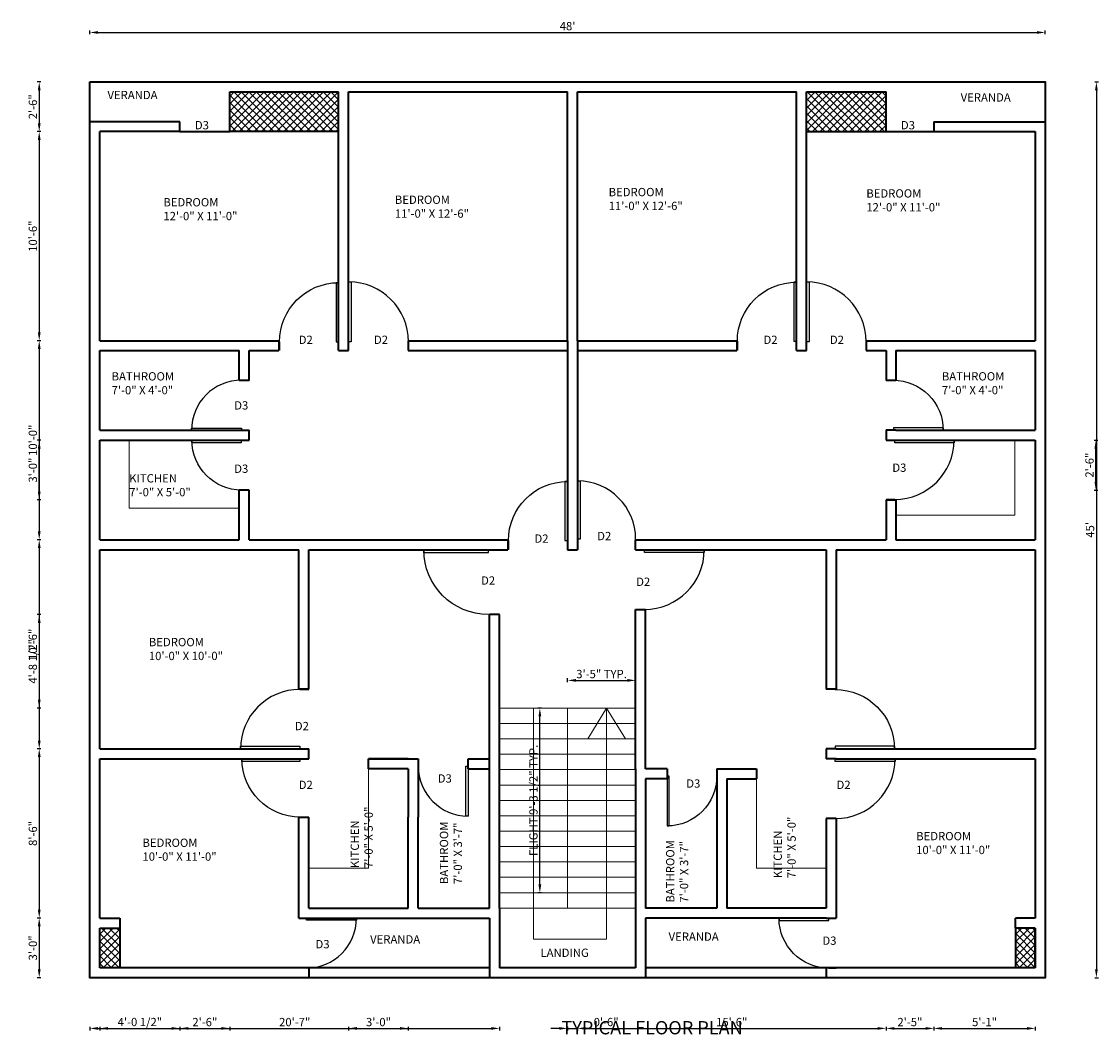
# Model space of a CAD drawing. Units: inches. Extents: x -42 to 607, y -560 to 51.
import ezdxf

# ---------------------------------------------------------------- set-up
doc = ezdxf.new("R2010")
doc.units = ezdxf.units.IN
for name, color, linetype, lineweight in [('A-ANNO-DIMS', 2, 'Continuous', 18), ('A-ANNO-SYMB', 7, 'Continuous', 18), ('A-ANNO-TEXT', 7, 'Continuous', 35), ('A-AREA-IDEN', 7, 'Continuous', 18), ('A-DOOR', 3, 'Continuous', 25), ('A-DOOR-IDEN', 3, 'Continuous', 18), ('A-FLOR-FIXT', 9, 'Continuous', 18), ('A-FLOR-STRS', 4, 'Continuous', 18), ('A-WALL', 7, 'Continuous', 35), ('A-WALL-PATT', 28, 'Continuous', 13)]:
    doc.layers.add(name, color=color, linetype=linetype, lineweight=lineweight)
doc.styles.get("Standard").update_dxf_attribs({"font": 'arial.ttf'})
doc.dimstyles.new('ISO-25', dxfattribs={"dimtxt": 5, "dimasz": 5, "dimexe": 1.25, "dimexo": 0.625, "dimtad": 1, "dimlunit": 3, "dimtxsty": 'Standard', "dimcen": 2.5, "dimadec": 0, "dimazin": 0, "dimtfac": 1, "dimtmove": 0, "dimatfit": 3, "dimfxl": 1, "dimfxlon": 1, "dimarcsym": 0})

# ---------------------------------------------------------------- blocks, each defined once
blk = doc.blocks.new('*U2')
for p, q in [((0, 0), (0, -6)), ((40, 0), (40, -6))]:
    blk.add_line(p, q)
blk.add_lwpolyline([(0, 0), (0, 40), (1.75, 40), (1.75, 0)], close=True)
blk.add_arc((0, 0), 40, 0, 90)
blk = doc.blocks.new('*D3')
at = {"layer": 'A-ANNO-DIMS', "color": 0, "lineweight": -2, "transparency": 16777216}
for p, q in [((-1, 43.9), (-1, 46.15)), ((575, 43.9), (575, 46.15)), ((4, 44.9), (570, 44.9))]:
    blk.add_line(p, q, dxfattribs=at)
at = {"layer": 'A-ANNO-DIMS', "color": 0, "transparency": 16777216}
for points in [[(4, 45.73), (4, 44.07), (-1, 44.9)], [(570, 45.73), (570, 44.07), (575, 44.9)]]:
    blk.add_solid(points, dxfattribs=at)
at = {"layer": 'Defpoints', "color": 0, "transparency": 16777216}
for p in [(575, 44.9), (-1, 15.11), (575, 15.11)]:
    blk.add_point(p, dxfattribs=at)
at = {"layer": 'A-ANNO-DIMS', "color": 0, "transparency": 16777216, "insert": (287, 48.08), "char_height": 5, "attachment_point": 5}
blk.add_mtext("48'", dxfattribs=at)
blk = doc.blocks.new('*D4')
at = {"layer": 'A-ANNO-DIMS', "color": 0, "lineweight": -2, "transparency": 16777216}
for p, q in [((604.84, 15.11), (607.09, 15.11)), ((605.84, 10.11), (605.84, -519.89)), ((604.84, -524.89), (607.09, -524.89))]:
    blk.add_line(p, q, dxfattribs=at)
at = {"layer": 'A-ANNO-DIMS', "color": 0, "transparency": 16777216}
for points in [[(605.01, 10.11), (606.67, 10.11), (605.84, 15.11)], [(605.01, -519.89), (606.67, -519.89), (605.84, -524.89)]]:
    blk.add_solid(points, dxfattribs=at)
at = {"layer": 'Defpoints', "color": 0, "transparency": 16777216}
for p in [(575, 15.11), (575, -524.89), (605.84, -524.89)]:
    blk.add_point(p, dxfattribs=at)
at = {"layer": 'A-ANNO-DIMS', "color": 0, "transparency": 16777216, "insert": (602.67, -254.89), "char_height": 5, "attachment_point": 5, "rotation": 90}
blk.add_mtext("45'", dxfattribs=at)
blk = doc.blocks.new('STAIR-FLIGHT-41IN')
for p, q in [((41, 111.29), (0, 111.29)), ((41, 102.01), (0, 102.01)), ((41, 92.74), (0, 92.74)), ((41, 83.46), (0, 83.46)), ((41, 74.19), (0, 74.19)), ((41, 64.92), (0, 64.92)), ((41, 55.64), (0, 55.64)), ((41, 46.37), (0, 46.37)), ((41, 37.1), (0, 37.1)), ((41, 27.82), (0, 27.82)), ((41, 18.55), (0, 18.55)), ((41, 9.27), (0, 9.27)), ((41, 0), (0, 0))]:
    blk.add_line(p, q)
blk = doc.blocks.new('*D6')
at = {"layer": 'A-ANNO-DIMS', "color": 0, "lineweight": -2, "transparency": 16777216}
for p, q in [((271.31, -362.33), (269.06, -362.33)), ((270.31, -468.61), (270.31, -367.33)), ((271.31, -473.61), (269.06, -473.61))]:
    blk.add_line(p, q, dxfattribs=at)
at = {"layer": 'A-ANNO-DIMS', "color": 0, "transparency": 16777216}
for points in [[(269.47, -367.33), (271.14, -367.33), (270.31, -362.33)], [(269.47, -468.61), (271.14, -468.61), (270.31, -473.61)]]:
    blk.add_solid(points, dxfattribs=at)
at = {"layer": 'Defpoints', "color": 0, "transparency": 16777216}
for p in [(270.31, -362.33), (287, -362.33), (287, -473.61)]:
    blk.add_point(p, dxfattribs=at)
at = {"layer": 'A-ANNO-DIMS', "color": 0, "transparency": 16777216, "insert": (267.1, -417.97), "char_height": 5, "attachment_point": 5, "rotation": 90}
blk.add_mtext('FLIGHT 9\'-3 1/2" TYP.', dxfattribs=at)
blk = doc.blocks.new('*D7')
at = {"layer": 'A-ANNO-DIMS', "color": 0, "lineweight": -2, "transparency": 16777216}
for p, q in [((287, -346.64), (287, -344.39)), ((292, -345.64), (323, -345.64)), ((328, -346.64), (328, -344.39))]:
    blk.add_line(p, q, dxfattribs=at)
at = {"layer": 'A-ANNO-DIMS', "color": 0, "transparency": 16777216}
for points in [[(292, -344.8), (292, -346.47), (287, -345.64)], [(323, -344.8), (323, -346.47), (328, -345.64)]]:
    blk.add_solid(points, dxfattribs=at)
at = {"layer": 'Defpoints', "color": 0, "transparency": 16777216}
for p in [(328, -345.64), (287, -362.33), (328, -362.33)]:
    blk.add_point(p, dxfattribs=at)
at = {"layer": 'A-ANNO-DIMS', "color": 0, "transparency": 16777216, "insert": (307.5, -342.46), "char_height": 5, "attachment_point": 5}
blk.add_mtext('3\'-5" TYP.', dxfattribs=at)
blk = doc.blocks.new('*D8')
at = {"layer": 'A-ANNO-DIMS', "color": 0, "lineweight": -2, "transparency": 16777216}
for p, q in [((-30.52, 15.11), (-32.77, 15.11)), ((-31.52, 10.11), (-31.52, -9.89)), ((-30.52, -14.89), (-32.77, -14.89))]:
    blk.add_line(p, q, dxfattribs=at)
at = {"layer": 'A-ANNO-DIMS', "color": 0, "transparency": 16777216}
for points in [[(-32.35, 10.11), (-30.69, 10.11), (-31.52, 15.11)], [(-32.35, -9.89), (-30.69, -9.89), (-31.52, -14.89)]]:
    blk.add_solid(points, dxfattribs=at)
at = {"layer": 'Defpoints', "color": 0, "transparency": 16777216}
for p in [(-1, 15.11), (-31.52, -14.89), (5, -14.89)]:
    blk.add_point(p, dxfattribs=at)
at = {"layer": 'A-ANNO-DIMS', "color": 0, "transparency": 16777216, "insert": (-34.7, 0.11), "char_height": 5, "attachment_point": 5, "rotation": 90}
blk.add_mtext('2\'-6"', dxfattribs=at)
blk = doc.blocks.new('*D9')
at = {"layer": 'A-ANNO-DIMS', "color": 0, "lineweight": -2, "transparency": 16777216}
for p, q in [((-30.52, -14.89), (-32.77, -14.89)), ((-31.52, -19.89), (-31.52, -135.89)), ((-30.52, -140.89), (-32.77, -140.89))]:
    blk.add_line(p, q, dxfattribs=at)
at = {"layer": 'A-ANNO-DIMS', "color": 0, "transparency": 16777216}
for points in [[(-32.35, -19.89), (-30.69, -19.89), (-31.52, -14.89)], [(-32.35, -135.89), (-30.69, -135.89), (-31.52, -140.89)]]:
    blk.add_solid(points, dxfattribs=at)
at = {"layer": 'Defpoints', "color": 0, "transparency": 16777216}
for p in [(5, -14.89), (-31.52, -140.89), (5, -140.89)]:
    blk.add_point(p, dxfattribs=at)
at = {"layer": 'A-ANNO-DIMS', "color": 0, "transparency": 16777216, "insert": (-34.7, -77.89), "char_height": 5, "attachment_point": 5, "rotation": 90}
blk.add_mtext('10\'-6"', dxfattribs=at)
blk = doc.blocks.new('*D10')
at = {"layer": 'A-ANNO-DIMS', "color": 0, "lineweight": -2, "transparency": 16777216}
for p, q in [((-30.52, -140.89), (-32.77, -140.89)), ((-31.52, -145.89), (-31.52, -255.89)), ((-30.52, -260.89), (-32.77, -260.89))]:
    blk.add_line(p, q, dxfattribs=at)
at = {"layer": 'A-ANNO-DIMS', "color": 0, "transparency": 16777216}
for points in [[(-32.35, -145.89), (-30.69, -145.89), (-31.52, -140.89)], [(-32.35, -255.89), (-30.69, -255.89), (-31.52, -260.89)]]:
    blk.add_solid(points, dxfattribs=at)
at = {"layer": 'Defpoints', "color": 0, "transparency": 16777216}
for p in [(5, -140.89), (-31.52, -260.89), (5, -260.89)]:
    blk.add_point(p, dxfattribs=at)
at = {"layer": 'A-ANNO-DIMS', "color": 0, "transparency": 16777216, "insert": (-34.7, -200.89), "char_height": 5, "attachment_point": 5, "rotation": 90}
blk.add_mtext('10\'-0"', dxfattribs=at)
blk = doc.blocks.new('*D11')
at = {"layer": 'A-ANNO-DIMS', "color": 0, "lineweight": -2, "transparency": 16777216}
for p, q in [((-30.52, -260.89), (-32.77, -260.89)), ((-31.52, -265.89), (-31.52, -381.89)), ((-30.52, -386.89), (-32.77, -386.89))]:
    blk.add_line(p, q, dxfattribs=at)
at = {"layer": 'A-ANNO-DIMS', "color": 0, "transparency": 16777216}
for points in [[(-32.35, -265.89), (-30.69, -265.89), (-31.52, -260.89)], [(-32.35, -381.89), (-30.69, -381.89), (-31.52, -386.89)]]:
    blk.add_solid(points, dxfattribs=at)
at = {"layer": 'Defpoints', "color": 0, "transparency": 16777216}
for p in [(5, -260.89), (-31.52, -386.89), (5, -386.89)]:
    blk.add_point(p, dxfattribs=at)
at = {"layer": 'A-ANNO-DIMS', "color": 0, "transparency": 16777216, "insert": (-34.7, -323.89), "char_height": 5, "attachment_point": 5, "rotation": 90}
blk.add_mtext('10\'-6"', dxfattribs=at)
blk = doc.blocks.new('*D12')
at = {"layer": 'A-ANNO-DIMS', "color": 0, "lineweight": -2, "transparency": 16777216}
for p, q in [((-30.52, -386.89), (-32.77, -386.89)), ((-31.52, -391.89), (-31.52, -483.89)), ((-30.52, -488.89), (-32.77, -488.89))]:
    blk.add_line(p, q, dxfattribs=at)
at = {"layer": 'A-ANNO-DIMS', "color": 0, "transparency": 16777216}
for points in [[(-32.35, -391.89), (-30.69, -391.89), (-31.52, -386.89)], [(-32.35, -483.89), (-30.69, -483.89), (-31.52, -488.89)]]:
    blk.add_solid(points, dxfattribs=at)
at = {"layer": 'Defpoints', "color": 0, "transparency": 16777216}
for p in [(5, -386.89), (-31.52, -488.89), (5, -488.89)]:
    blk.add_point(p, dxfattribs=at)
at = {"layer": 'A-ANNO-DIMS', "color": 0, "transparency": 16777216, "insert": (-34.7, -437.89), "char_height": 5, "attachment_point": 5, "rotation": 90}
blk.add_mtext('8\'-6"', dxfattribs=at)
blk = doc.blocks.new('*D13')
at = {"layer": 'A-ANNO-DIMS', "color": 0, "lineweight": -2, "transparency": 16777216}
for p, q in [((-30.52, -488.89), (-32.77, -488.89)), ((-31.52, -493.89), (-31.52, -519.89)), ((-30.52, -524.89), (-32.77, -524.89))]:
    blk.add_line(p, q, dxfattribs=at)
at = {"layer": 'A-ANNO-DIMS', "color": 0, "transparency": 16777216}
for points in [[(-32.35, -493.89), (-30.69, -493.89), (-31.52, -488.89)], [(-32.35, -519.89), (-30.69, -519.89), (-31.52, -524.89)]]:
    blk.add_solid(points, dxfattribs=at)
at = {"layer": 'Defpoints', "color": 0, "transparency": 16777216}
for p in [(5, -488.89), (-31.52, -524.89), (-1, -524.89)]:
    blk.add_point(p, dxfattribs=at)
at = {"layer": 'A-ANNO-DIMS', "color": 0, "transparency": 16777216, "insert": (-34.7, -506.89), "char_height": 5, "attachment_point": 5, "rotation": 90}
blk.add_mtext('3\'-0"', dxfattribs=at)
blk = doc.blocks.new('*D14')
at = {"layer": 'A-ANNO-DIMS', "color": 0, "lineweight": -2, "transparency": 16777216}
for p, q in [((-1, -554.41), (-1, -556.66)), ((4, -555.41), (241, -555.41)), ((246, -554.41), (246, -556.66))]:
    blk.add_line(p, q, dxfattribs=at)
at = {"layer": 'A-ANNO-DIMS', "color": 0, "transparency": 16777216}
for points in [[(4, -554.58), (4, -556.24), (-1, -555.41)], [(241, -554.58), (241, -556.24), (246, -555.41)]]:
    blk.add_solid(points, dxfattribs=at)
at = {"layer": 'Defpoints', "color": 0, "transparency": 16777216}
for p in [(246, -518.89), (-1, -524.89), (246, -555.41)]:
    blk.add_point(p, dxfattribs=at)
at = {"layer": 'A-ANNO-DIMS', "color": 0, "transparency": 16777216, "insert": (122.5, -552.23), "char_height": 5, "attachment_point": 5}
blk.add_mtext('20\'-7"', dxfattribs=at)
blk = doc.blocks.new('*D15')
at = {"layer": 'A-ANNO-DIMS', "color": 0, "lineweight": -2, "transparency": 16777216}
for p, q in [((-30.52, -306.02), (-32.77, -306.02)), ((-31.52, -311.02), (-31.52, -357.33)), ((-30.52, -362.33), (-32.77, -362.33))]:
    blk.add_line(p, q, dxfattribs=at)
at = {"layer": 'A-ANNO-DIMS', "color": 0, "transparency": 16777216}
for points in [[(-32.35, -311.02), (-30.69, -311.02), (-31.52, -306.02)], [(-32.35, -357.33), (-30.69, -357.33), (-31.52, -362.33)]]:
    blk.add_solid(points, dxfattribs=at)
at = {"layer": 'Defpoints', "color": 0, "transparency": 16777216}
for p in [(240, -306.02), (-31.52, -362.33), (246, -362.33)]:
    blk.add_point(p, dxfattribs=at)
at = {"layer": 'A-ANNO-DIMS', "color": 0, "transparency": 16777216, "insert": (-34.73, -334.17), "char_height": 5, "attachment_point": 5, "rotation": 90}
blk.add_mtext('4\'-8 1/2"', dxfattribs=at)
blk = doc.blocks.new('*D16')
at = {"layer": 'A-ANNO-DIMS', "color": 0, "lineweight": -2, "transparency": 16777216}
for p, q in [((5, -554.41), (5, -556.66)), ((10, -555.41), (48.34, -555.41)), ((53.34, -554.41), (53.34, -556.66))]:
    blk.add_line(p, q, dxfattribs=at)
at = {"layer": 'A-ANNO-DIMS', "color": 0, "transparency": 16777216}
for points in [[(10, -554.58), (10, -556.24), (5, -555.41)], [(48.34, -554.58), (48.34, -556.24), (53.34, -555.41)]]:
    blk.add_solid(points, dxfattribs=at)
at = {"layer": 'Defpoints', "color": 0, "transparency": 16777216}
for p in [(5, -14.89), (53.34, -14.89), (53.34, -555.41)]:
    blk.add_point(p, dxfattribs=at)
at = {"layer": 'A-ANNO-DIMS', "color": 0, "transparency": 16777216, "insert": (29.17, -552.2), "char_height": 5, "attachment_point": 5}
blk.add_mtext('4\'-0 1/2"', dxfattribs=at)
blk = doc.blocks.new('*D17')
at = {"layer": 'A-ANNO-DIMS', "color": 0, "lineweight": -2, "transparency": 16777216}
for p, q in [((53.34, -554.41), (53.34, -556.66)), ((58.34, -555.41), (78.34, -555.41)), ((83.34, -554.41), (83.34, -556.66))]:
    blk.add_line(p, q, dxfattribs=at)
at = {"layer": 'A-ANNO-DIMS', "color": 0, "transparency": 16777216}
for points in [[(58.34, -554.58), (58.34, -556.24), (53.34, -555.41)], [(78.34, -554.58), (78.34, -556.24), (83.34, -555.41)]]:
    blk.add_solid(points, dxfattribs=at)
at = {"layer": 'Defpoints', "color": 0, "transparency": 16777216}
for p in [(53.34, -14.89), (83.34, -14.89), (83.34, -555.41)]:
    blk.add_point(p, dxfattribs=at)
at = {"layer": 'A-ANNO-DIMS', "color": 0, "transparency": 16777216, "insert": (68.34, -552.23), "char_height": 5, "attachment_point": 5}
blk.add_mtext('2\'-6"', dxfattribs=at)
blk = doc.blocks.new('*D18')
at = {"layer": 'A-ANNO-DIMS', "color": 0, "lineweight": -2, "transparency": 16777216}
for p, q in [((507.85, -554.41), (507.85, -556.66)), ((512.85, -555.41), (564, -555.41)), ((569, -554.41), (569, -556.66))]:
    blk.add_line(p, q, dxfattribs=at)
at = {"layer": 'A-ANNO-DIMS', "color": 0, "transparency": 16777216}
for points in [[(512.85, -554.58), (512.85, -556.24), (507.85, -555.41)], [(564, -554.58), (564, -556.24), (569, -555.41)]]:
    blk.add_solid(points, dxfattribs=at)
at = {"layer": 'Defpoints', "color": 0, "transparency": 16777216}
for p in [(507.85, -14.89), (569, -14.89), (569, -555.41)]:
    blk.add_point(p, dxfattribs=at)
at = {"layer": 'A-ANNO-DIMS', "color": 0, "transparency": 16777216, "insert": (538.42, -552.23), "char_height": 5, "attachment_point": 5}
blk.add_mtext('5\'-1"', dxfattribs=at)
blk = doc.blocks.new('*D19')
at = {"layer": 'A-ANNO-DIMS', "color": 0, "lineweight": -2, "transparency": 16777216}
for p, q in [((479, -554.41), (479, -556.66)), ((484, -555.41), (502.85, -555.41)), ((507.85, -554.41), (507.85, -556.66))]:
    blk.add_line(p, q, dxfattribs=at)
at = {"layer": 'A-ANNO-DIMS', "color": 0, "transparency": 16777216}
for points in [[(484, -554.58), (484, -556.24), (479, -555.41)], [(502.85, -554.58), (502.85, -556.24), (507.85, -555.41)]]:
    blk.add_solid(points, dxfattribs=at)
at = {"layer": 'Defpoints', "color": 0, "transparency": 16777216}
for p in [(479, -14.89), (507.85, -14.89), (507.85, -555.41)]:
    blk.add_point(p, dxfattribs=at)
at = {"layer": 'A-ANNO-DIMS', "color": 0, "transparency": 16777216, "insert": (493.42, -552.23), "char_height": 5, "attachment_point": 5}
blk.add_mtext('2\'-5"', dxfattribs=at)
blk = doc.blocks.new('*D20')
at = {"layer": 'A-ANNO-DIMS', "color": 0, "lineweight": -2, "transparency": 16777216}
for p, q in [((155, -554.41), (155, -556.66)), ((160, -555.41), (186, -555.41)), ((191, -554.41), (191, -556.66))]:
    blk.add_line(p, q, dxfattribs=at)
at = {"layer": 'A-ANNO-DIMS', "color": 0, "transparency": 16777216}
for points in [[(160, -554.58), (160, -556.24), (155, -555.41)], [(186, -554.58), (186, -556.24), (191, -555.41)]]:
    blk.add_solid(points, dxfattribs=at)
at = {"layer": 'Defpoints', "color": 0, "transparency": 16777216}
for p in [(155, -146.89), (191, -146.89), (191, -555.41)]:
    blk.add_point(p, dxfattribs=at)
at = {"layer": 'A-ANNO-DIMS', "color": 0, "transparency": 16777216, "insert": (173, -552.23), "char_height": 5, "attachment_point": 5}
blk.add_mtext('3\'-0"', dxfattribs=at)
blk = doc.blocks.new('*D21')
at = {"layer": 'A-ANNO-DIMS', "color": 0, "lineweight": -2, "transparency": 16777216}
for p, q in [((282, -555.41), (277, -555.41)), ((287, -554.41), (287, -556.66)), ((287, -555.41), (293, -555.41)), ((293, -554.41), (293, -556.66)), ((298, -555.41), (317.54, -555.41))]:
    blk.add_line(p, q, dxfattribs=at)
at = {"layer": 'A-ANNO-DIMS', "color": 0, "transparency": 16777216}
for points in [[(282, -554.58), (282, -556.24), (287, -555.41)], [(298, -554.58), (298, -556.24), (293, -555.41)]]:
    blk.add_solid(points, dxfattribs=at)
at = {"layer": 'Defpoints', "color": 0, "transparency": 16777216}
for p in [(287, -266.89), (293, -266.89), (293, -555.41)]:
    blk.add_point(p, dxfattribs=at)
at = {"layer": 'A-ANNO-DIMS', "color": 0, "transparency": 16777216, "insert": (310.27, -552.23), "char_height": 5, "attachment_point": 5}
blk.add_mtext('0\'-6"', dxfattribs=at)
blk = doc.blocks.new('*D22')
at = {"layer": 'A-ANNO-DIMS', "color": 0, "lineweight": -2, "transparency": 16777216}
for p, q in [((604.52, -200.89), (606.77, -200.89)), ((605.52, -225.89), (605.52, -205.89)), ((604.52, -230.89), (606.77, -230.89))]:
    blk.add_line(p, q, dxfattribs=at)
at = {"layer": 'A-ANNO-DIMS', "color": 0, "transparency": 16777216}
for points in [[(604.69, -205.89), (606.35, -205.89), (605.52, -200.89)], [(604.69, -225.89), (606.35, -225.89), (605.52, -230.89)]]:
    blk.add_solid(points, dxfattribs=at)
at = {"layer": 'Defpoints', "color": 0, "transparency": 16777216}
for p in [(95, -200.89), (605.52, -200.89), (95, -230.89)]:
    blk.add_point(p, dxfattribs=at)
at = {"layer": 'A-ANNO-DIMS', "color": 0, "transparency": 16777216, "insert": (602.34, -215.89), "char_height": 5, "attachment_point": 5, "rotation": 90}
blk.add_mtext('2\'-6"', dxfattribs=at)
blk = doc.blocks.new('*D23')
at = {"layer": 'A-ANNO-DIMS', "color": 0, "lineweight": -2, "transparency": 16777216}
for p, q in [((-30.52, -200.89), (-32.77, -200.89)), ((-31.52, -231.89), (-31.52, -205.89)), ((-30.52, -236.89), (-32.77, -236.89))]:
    blk.add_line(p, q, dxfattribs=at)
at = {"layer": 'A-ANNO-DIMS', "color": 0, "transparency": 16777216}
for points in [[(-32.35, -205.89), (-30.69, -205.89), (-31.52, -200.89)], [(-32.35, -231.89), (-30.69, -231.89), (-31.52, -236.89)]]:
    blk.add_solid(points, dxfattribs=at)
at = {"layer": 'Defpoints', "color": 0, "transparency": 16777216}
for p in [(-31.52, -200.89), (479, -200.89), (479, -236.89)]:
    blk.add_point(p, dxfattribs=at)
at = {"layer": 'A-ANNO-DIMS', "color": 0, "transparency": 16777216, "insert": (-34.7, -218.89), "char_height": 5, "attachment_point": 5, "rotation": 90}
blk.add_mtext('3\'-0"', dxfattribs=at)
blk = doc.blocks.new('*D24')
at = {"layer": 'A-ANNO-DIMS', "color": 0, "lineweight": -2, "transparency": 16777216}
for p, q in [((293, -554.41), (293, -556.66)), ((298, -555.41), (474, -555.41)), ((479, -554.41), (479, -556.66))]:
    blk.add_line(p, q, dxfattribs=at)
at = {"layer": 'A-ANNO-DIMS', "color": 0, "transparency": 16777216}
for points in [[(298, -554.58), (298, -556.24), (293, -555.41)], [(474, -554.58), (474, -556.24), (479, -555.41)]]:
    blk.add_solid(points, dxfattribs=at)
at = {"layer": 'Defpoints', "color": 0, "transparency": 16777216}
for p in [(293, -146.89), (479, -146.89), (479, -555.41)]:
    blk.add_point(p, dxfattribs=at)
at = {"layer": 'A-ANNO-DIMS', "color": 0, "transparency": 16777216, "insert": (386, -552.23), "char_height": 5, "attachment_point": 5}
blk.add_mtext('15\'-6"', dxfattribs=at)

msp = doc.modelspace()

# ---------------------------------------------------------------- hatches: boundary and pattern name
at = {"layer": 'A-WALL-PATT'}
h = msp.add_hatch(dxfattribs=at)
h.set_pattern_fill('ANSI37', color=256)
h.set_pattern_definition([(45, (-156.5172, 2e-14), (-2.245064, 2.245064), []), (135, (-156.5172, 2e-14), (-2.245064, -2.245064), [])])
h.paths.add_polyline_path([(17, -494.888), (5, -494.888), (5, -518.888), (17, -518.888)])
h.paths.add_polyline_path([(569, -494.888), (557, -494.888), (557, -518.888), (569, -518.888)])
h.paths.add_polyline_path([(479, 9.112), (431, 9.112), (431, -14.888), (479, -14.888)])
h.paths.add_polyline_path([(149, 9.112), (83.336, 9.112), (83.336, -8.888), (83.336, -14.888), (149, -14.888)])

# ---------------------------------------------------------------- linework, layer by layer
at = {"layer": 'A-ANNO-SYMB'}
for p, q in [((266.5, -362.329), (266.5, -501.605)), ((310.468, -362.329), (299.202, -380.877)), ((310.468, -501.605), (310.468, -362.329)), ((310.468, -362.329), (321.981, -380.877)), ((266.5, -501.605), (310.468, -501.605))]:
    msp.add_line(p, q, dxfattribs=at)
at = {"layer": 'A-FLOR-FIXT'}
for p, q in [((22.754, -241.785), (22.754, -200.888)), ((556.59, -246.142), (556.59, -200.888)), ((89, -241.785), (22.754, -241.785)), ((485, -246.142), (556.59, -246.142)), ((167, -398.888), (167, -458.888)), ((401, -404.888), (401, -458.888)), ((131, -458.888), (167, -458.888)), ((443, -458.888), (401, -458.888))]:
    msp.add_line(p, q, dxfattribs=at)
at = {"layer": 'A-FLOR-STRS'}
for p, q in [((287, -482.888), (287, -362.329)), ((328, -482.888), (246, -482.888)), ((287, -482.888), (246, -482.888))]:
    msp.add_line(p, q, dxfattribs=at)
at = {"layer": 'A-WALL'}
for p, q in [((83.336, 9.112), (149, 9.112)), ((83.336, -8.888), (83.336, 9.112)), ((149, -146.888), (149, 9.112)), ((155, -146.888), (155, 9.112)), ((155, 9.112), (287, 9.112)), ((287, -140.888), (287, 9.112)), ((293, -140.888), (293, 9.112)), ((293, 9.112), (425, 9.112)), ((425, -146.888), (425, 9.112)), ((431, -146.888), (431, 9.112)), ((431, 9.112), (479, 9.112)), ((479, -14.888), (479, 9.112)), ((5, -8.888), (-1, -8.888)), ((53.336, -8.888), (5, -8.888)), ((53.336, -14.888), (53.336, -8.888)), ((83.336, -14.888), (83.336, -8.888)), ((507.846, -8.888), (569, -8.888)), ((507.846, -8.888), (507.846, -14.888)), ((569, -8.888), (575, -8.888)), ((5, -140.888), (5, -14.888)), ((53.336, -14.888), (5, -14.888)), ((53.336, -14.888), (83.336, -14.888)), ((149, -14.888), (83.336, -14.888)), ((431, -14.888), (569, -14.888)), ((569, -14.888), (569, -140.888)), ((5, -140.888), (113, -140.888)), ((113, -140.888), (113, -146.888)), ((191, -140.888), (287, -140.888)), ((191, -140.888), (191, -146.888)), ((287, -140.888), (287, -266.888)), ((293, -140.888), (389, -140.888)), ((293, -140.888), (293, -266.888)), ((389, -140.888), (389, -146.888)), ((467, -140.888), (569, -140.888)), ((467, -140.888), (467, -146.888)), ((5, -146.888), (89, -146.888)), ((5, -194.888), (5, -146.888)), ((89, -164.888), (89, -146.888)), ((95, -164.888), (95, -146.888)), ((95, -146.888), (113, -146.888)), ((149, -146.888), (155, -146.888)), ((191, -146.888), (287, -146.888)), ((293, -146.888), (389, -146.888)), ((425, -146.888), (431, -146.888)), ((467, -146.888), (479, -146.888)), ((479, -146.888), (479, -164.888)), ((485, -146.888), (485, -164.888)), ((485, -146.888), (569, -146.888)), ((569, -146.888), (569, -194.888)), ((95, -164.888), (89, -164.888)), ((485, -164.888), (479, -164.888)), ((5, -194.888), (95, -194.888)), ((5, -200.888), (95, -200.888)), ((5, -260.888), (5, -200.888)), ((95, -200.888), (95, -194.888)), ((479, -194.888), (479, -200.888)), ((485, -194.888), (479, -194.888)), ((479, -200.888), (569, -200.888)), ((485, -194.888), (569, -194.888)), ((569, -200.888), (569, -260.888)), ((89, -260.888), (89, -230.888)), ((95, -230.888), (89, -230.888)), ((95, -260.888), (95, -230.888)), ((479, -236.888), (479, -260.888)), ((479, -236.888), (485, -236.888)), ((485, -236.888), (485, -260.888)), ((5, -260.888), (89, -260.888)), ((95, -260.888), (113, -260.888)), ((113, -260.888), (240, -260.888)), ((240, -260.888), (251, -260.888)), ((251, -260.888), (251, -266.888)), ((328, -260.888), (479, -260.888)), ((328, -266.888), (328, -260.888)), ((485, -260.888), (569, -260.888)), ((5, -266.888), (113, -266.888)), ((5, -386.888), (5, -266.888)), ((113, -266.888), (125, -266.888)), ((125, -350.888), (125, -266.888)), ((131, -266.888), (240, -266.888)), ((131, -350.888), (131, -266.888)), ((234.805, -266.888), (251, -266.888)), ((287, -266.888), (293, -266.888)), ((328, -266.888), (443, -266.888)), ((443, -266.888), (443, -350.888)), ((449, -266.888), (449, -350.888)), ((449, -266.888), (569, -266.888)), ((569, -266.888), (569, -386.888)), ((328, -398.888), (328, -302.888)), ((328, -302.888), (334, -302.888)), ((334, -398.888), (334, -302.888)), ((240, -428.17), (240, -306.02)), ((246, -306.02), (240, -306.02)), ((246, -428.17), (246, -306.02)), ((131, -350.888), (125, -350.888)), ((449, -350.888), (443, -350.888)), ((5, -386.888), (131, -386.888)), ((131, -392.888), (131, -386.888)), ((449, -386.888), (443, -386.888)), ((443, -386.888), (443, -392.888)), ((449, -386.888), (569, -386.888)), ((5, -392.888), (131, -392.888)), ((5, -488.888), (5, -392.888)), ((191, -392.888), (167, -392.888)), ((167, -392.888), (197, -392.888)), ((167, -398.888), (167, -392.888)), ((197, -392.888), (197, -428.17)), ((227, -392.888), (240, -392.888)), ((227, -398.888), (227, -392.888)), ((240, -399.381), (240, -392.888)), ((449, -392.888), (443, -392.888)), ((449, -392.888), (569, -392.888)), ((569, -392.888), (569, -488.888)), ((191, -398.888), (167, -398.888)), ((191, -398.888), (191, -428.17)), ((227, -398.888), (240, -398.888)), ((328, -398.888), (328, -428.888)), ((347, -398.888), (334, -398.888)), ((347, -398.888), (347, -404.888)), ((377, -398.888), (377, -428.888)), ((377, -398.888), (401, -398.888)), ((401, -398.888), (401, -404.888)), ((334, -404.888), (334, -428.888)), ((347, -404.888), (334, -404.888)), ((383, -404.888), (383, -428.888)), ((383, -404.888), (401, -404.888)), ((125, -428.17), (131, -428.17)), ((125, -488.888), (125, -428.17)), ((131, -482.888), (131, -428.17)), ((191, -482.888), (191, -428.17)), ((197, -482.888), (197, -428.17)), ((240, -482.888), (240, -428.17)), ((246, -482.888), (246, -428.17)), ((328, -428.888), (328, -482.888)), ((334, -428.888), (334, -482.888)), ((377, -428.888), (377, -482.888)), ((383, -428.888), (383, -482.888)), ((443, -428.888), (443, -482.888)), ((449, -428.888), (443, -428.888)), ((449, -428.888), (449, -488.888)), ((131, -482.888), (191, -482.888)), ((197, -482.888), (240, -482.888)), ((246, -482.888), (246, -518.888)), ((328, -482.888), (328, -518.888)), ((377, -482.888), (334, -482.888)), ((443, -482.888), (383, -482.888)), ((5, -488.888), (17, -488.888)), ((17, -488.888), (17, -494.888)), ((125, -488.888), (131, -488.888)), ((131, -488.888), (240, -488.888)), ((240, -488.888), (240, -518.888)), ((443, -488.888), (334, -488.888)), ((334, -488.888), (334, -524.888)), ((443, -488.888), (449, -488.888)), ((569, -488.888), (557, -488.888)), ((557, -494.888), (557, -488.888)), ((5, -518.888), (5, -494.888)), ((5, -494.888), (17, -494.888)), ((17, -494.888), (17, -518.888)), ((569, -494.888), (557, -494.888)), ((557, -494.888), (557, -518.888)), ((569, -518.888), (569, -494.888)), ((569, -494.888), (569, -518.888)), ((240, -518.888), (5, -518.888)), ((131, -518.888), (131, -524.888)), ((240, -518.888), (240, -524.888)), ((328, -518.888), (246, -518.888)), ((569, -518.888), (334, -518.888)), ((443, -518.888), (443, -524.888))]:
    msp.add_line(p, q, dxfattribs=at)
msp.add_lwpolyline([(-1, 15.112), (575, 15.112), (575, -524.888), (-1, -524.888)], close=True, dxfattribs=at)

# ---------------------------------------------------------------- block references
at = {"layer": 'A-DOOR'}
for p, xscale, yscale, zscale in [((149, -141.545), -0.8906414144177713, 0.8906414144177713, 0.8906414144177713), ((155, -141.48), 0.9014412016206881, 0.9014412016206881, 0.9014412016206881), ((425, -141.213), -0.8906414144177713, 0.8906414144177713, 0.8906414144177713), ((431, -141.48), 0.9014412016206881, 0.9014412016206881, 0.9014412016206881), ((286.949, -261.385), -0.8906414144177713, 0.8906414144177713, 0.8906414144177713), ((293, -260.487), 0.8762992287586572, 0.8762992287586572, 0.8762992287586572)]:
    msp.add_blockref('*U2', p, dxfattribs=dict(at, xscale=xscale, yscale=yscale, zscale=zscale))
for p, xscale, yscale, zscale, rotation in [((90.465, -194.888), 0.7558047034111338, 0.7558047034111338, 0.7558047034111338, 90), ((483.463, -194.766), -0.7500117927487225, 0.7500117927487225, 0.7500117927487225, 270.0000000000001), ((90.5, -200.888), -0.7500117927487225, 0.7500117927487225, 0.7500117927487225, 90), ((484.348, -200.888), 0.8913673782740719, 0.8913673782740719, 0.8913673782740719, 270), ((239.296, -266.888), -0.975329866738669, 0.975329866738669, 0.975329866738669, 90), ((333.403, -266.888), 0.900534406420834, 0.900534406420834, 0.900534406420834, 270), ((125.631, -386.888), 0.8948649869026692, 0.8948649869026692, 0.8948649869026692, 90), ((448.364, -386.888), -0.8939931169519822, 0.8939931169519822, 0.8939931169519822, 270), ((125.736, -392.888), -0.8773008235321261, 0.8773008235321261, 0.8773008235321261, 90), ((227, -397.389), 0.7500117927487225, 0.7500117927487225, 0.7500117927487225, 180), ((448.448, -392.851), 0.9022238422237986, 0.9022238422237986, 0.9022238422237986, 270), ((347, -403.389), -0.7500117927487225, 0.7500117927487225, 0.7500117927487225, 180), ((129.535, -488.888), 0.7558047034111338, 0.7558047034111338, 0.7558047034111338, 270), ((444.5, -489.023), -0.7500117927487225, 0.7500117927487225, 0.7500117927487225, 90)]:
    msp.add_blockref('*U2', p, dxfattribs=dict(at, xscale=xscale, yscale=yscale, zscale=zscale, rotation=rotation))
at = {"layer": 'A-FLOR-STRS'}
for p in [(246, -473.615), (287, -473.615)]:
    msp.add_blockref('STAIR-FLIGHT-41IN', p, dxfattribs=at)

# ---------------------------------------------------------------- texts
at = {"layer": 'A-ANNO-TEXT', "insert": (283.308, -550.99), "char_height": 8, "attachment_point": 1}
msp.add_mtext_dynamic_manual_height_columns('TYPICAL FLOOR PLAN', width=290.8071, gutter_width=12.5, heights=[0], dxfattribs=at)
at = {"layer": 'A-AREA-IDEN', "char_height": 5, "attachment_point": 1}
for s, width, insert in [('VERANDA', 44.90641, (9.62, 9.709)), ('VERANDA', 27.17778, (524.015, 8.235)), ('BEDROOM\\P11\'-0" X 12\'-6"', 72.28337, (311.792, -48.812)), ('BEDROOM\\P12\'-0" X 11\'-0"', 100.92398, (467.136, -49.621)), ('BEDROOM\\P12\'-0" X 11\'-0"', 96.567, (43.325, -54.934)), ('BEDROOM\\P11\'-0" X 12\'-6"', 85.82722, (182.905, -53.423)), ('BATHROOM\\P7\'-0" X 4\'-0"', 47.31804, (12.126, -159.866)), ('BATHROOM\\P7\'-0" X 4\'-0"', 45.60833, (512.686, -159.859)), ('KITCHEN\\P7\'-0" X 5\'-0"', 38.71476, (22.754, -221.337)), ('BEDROOM\\P10\'-0" X 10\'-0"', 84.03829, (34.58, -320.065)), ('BEDROOM\\P10\'-0" X 11\'-0"', 79.99233, (30.731, -440.999)), ('BEDROOM\\P10\'-0" X 11\'-0"', 53.27342, (497.184, -437.008)), ('VERANDA', 62.28877, (167.969, -499.232)), ('VERANDA', 59.4223, (347.92, -497.588)), ('LANDING', 58.70359, (270.685, -507.318))]:
    msp.add_mtext_dynamic_manual_height_columns(s, width=width, gutter_width=12.5, heights=[0], dxfattribs=dict(at, insert=insert))
at = {"layer": 'A-AREA-IDEN', "char_height": 5, "attachment_point": 1, "rotation": 90}
for s, width, insert in [('KITCHEN\\P7\'-0" X 5\'-0"', 38.95443, (156.241, -458.764)), ('KITCHEN\\P7\'-0" X 5\'-0"', 38.95443, (411.241, -464.888)), ('BATHROOM\\P7\'-0" X 3\'-7"', 45.60833, (210.024, -468.416)), ('BATHROOM\\P7\'-0" X 3\'-7"', 45.60833, (346.41, -479.569))]:
    msp.add_mtext_dynamic_manual_height_columns(s, width=width, gutter_width=12.5, heights=[0], dxfattribs=dict(at, insert=insert))
at = {"layer": 'A-DOOR-IDEN', "char_height": 5, "attachment_point": 1}
for s, width, insert in [('D3', 10.15667, (62.312, -8.491)), ('D3', 10.15667, (487.972, -8.491)), ('D2', 28.39792, (124.934, -137.847)), ('D2', 28.39792, (170.273, -137.847)), ('D2', 28.39792, (405.136, -137.847)), ('D2', 28.39792, (445.164, -137.847)), ('D3', 10.15667, (86.042, -177.381)), ('D3', 10.15667, (86.042, -215.55)), ('D3', 10.15667, (482.825, -214.93)), ('D2', 28.39792, (267.059, -257.669)), ('D2', 28.39792, (304.869, -256.137)), ('D2', 28.39792, (234.87, -282.941)), ('D2', 28.39792, (328.372, -283.706)), ('D2', 28.39792, (122.585, -370.661)), ('D3', 10.15667, (208.752, -402.253)), ('D2', 28.39792, (124.934, -406.09)), ('D3', 10.15667, (358.58, -405.308)), ('D2', 28.39792, (449.18, -406.103)), ('D3', 10.15667, (440.68, -500.016)), ('D3', 10.15667, (135.048, -502.128))]:
    msp.add_mtext_dynamic_manual_height_columns(s, width=width, gutter_width=12.5, heights=[0], dxfattribs=dict(at, insert=insert))

# ---------------------------------------------------------------- dimensions: what is measured, and where the dimension line sits
at = {"layer": 'A-ANNO-DIMS'}
dim = msp.add_linear_dim(base=(575, 44.898), p1=(-1, 15.112), p2=(575, 15.112), dimstyle='ISO-25', override={"dimclrd": 0, "dimclre": 0, "dimclrt": 0}, dxfattribs=at)
dim.commit()
dim.dimension.update_dxf_attribs({"geometry": '*D3', "text_midpoint": (287, 44.898), "dimtype": 160})
for base, p1, p2, override, picture, middle in [((-31.52, -14.888), (-1, 15.112), (5, -14.888), {"dimdec": 1, "dimlfac": 1, "dimrnd": 0, "dimzin": 1, "dimdsep": 46, "dimlunit": 4, "dimfrac": 2}, '*D8', (-34.698, 0.112)), ((605.839, -524.888), (575, 15.112), (575, -524.888), {"dimclrd": 0, "dimclre": 0, "dimclrt": 0}, '*D4', (602.671, -254.888)), ((-31.52, -140.888), (5, -14.888), (5, -140.888), {"dimdec": 1, "dimlfac": 1, "dimrnd": 0, "dimzin": 1, "dimdsep": 46, "dimlunit": 4, "dimfrac": 2}, '*D9', (-34.698, -77.888)), ((-31.52, -260.888), (5, -140.888), (5, -260.888), {"dimdec": 1, "dimlfac": 1, "dimrnd": 0, "dimzin": 1, "dimdsep": 46, "dimlunit": 4, "dimfrac": 2}, '*D10', (-34.698, -200.888)), ((-31.52, -200.888), (479, -236.888), (479, -200.888), {"dimdec": 1, "dimlfac": 1, "dimrnd": 0, "dimzin": 1, "dimdsep": 46, "dimlunit": 4, "dimfrac": 2}, '*D23', (-34.7, -218.888)), ((605.52, -200.888), (95, -230.889), (95, -200.888), {"dimdec": 1, "dimlfac": 1, "dimrnd": 0, "dimzin": 1, "dimdsep": 46, "dimlunit": 4, "dimfrac": 2}, '*D22', (602.342, -215.889)), ((-31.52, -386.888), (5, -260.888), (5, -386.888), {"dimdec": 1, "dimlfac": 1, "dimrnd": 0, "dimzin": 1, "dimdsep": 46, "dimlunit": 4, "dimfrac": 2}, '*D11', (-34.698, -323.888)), ((-31.52, -362.329), (240, -306.02), (246, -362.329), {"dimdec": 1, "dimlfac": 1, "dimrnd": 0, "dimzin": 1, "dimdsep": 46, "dimlunit": 4, "dimfrac": 2}, '*D15', (-34.73, -334.174)), ((-31.52, -488.888), (5, -386.888), (5, -488.888), {"dimdec": 1, "dimlfac": 1, "dimrnd": 0, "dimzin": 1, "dimdsep": 46, "dimlunit": 4, "dimfrac": 2}, '*D12', (-34.698, -437.888)), ((-31.52, -524.888), (5, -488.888), (-1, -524.888), {"dimdec": 1, "dimlfac": 1, "dimrnd": 0, "dimzin": 1, "dimdsep": 46, "dimlunit": 4, "dimfrac": 2}, '*D13', (-34.7, -506.888))]:
    dim = msp.add_linear_dim(base=base, p1=p1, p2=p2, angle=90, dimstyle='ISO-25', override=override, dxfattribs=at)
    dim.commit()
    dim.dimension.update_dxf_attribs({"geometry": picture, "text_midpoint": middle})
for base, p1, p2, picture, middle in [((53.336, -555.408), (5, -14.888), (53.336, -14.888), '*D16', (29.168, -552.198)), ((83.336, -555.408), (53.336, -14.888), (83.336, -14.888), '*D17', (68.336, -552.231)), ((507.846, -555.408), (479, -14.888), (507.846, -14.888), '*D19', (493.423, -552.231)), ((569, -555.408), (507.846, -14.888), (569, -14.888), '*D18', (538.423, -552.231)), ((191, -555.408), (155, -146.888), (191, -146.888), '*D20', (173, -552.229)), ((479, -555.408), (293, -146.888), (479, -146.888), '*D24', (386, -552.231)), ((293, -555.408), (287, -266.888), (293, -266.888), '*D21', (310.271, -552.231)), ((246, -555.408), (-1, -524.888), (246, -518.888), '*D14', (122.5, -552.231))]:
    dim = msp.add_linear_dim(base=base, p1=p1, p2=p2, dimstyle='ISO-25', override={"dimdec": 1, "dimlfac": 1, "dimrnd": 0, "dimzin": 1, "dimdsep": 46, "dimlunit": 4, "dimfrac": 2}, dxfattribs=at)
    dim.commit()
    dim.dimension.update_dxf_attribs({"geometry": picture, "text_midpoint": middle})
dim = msp.add_linear_dim(base=(328, -345.636), p1=(287, -362.329), p2=(328, -362.329), text='<> TYP.', dimstyle='ISO-25', override={"dimdec": 1, "dimlfac": 1, "dimrnd": 0, "dimzin": 1, "dimdsep": 46, "dimlunit": 4, "dimfrac": 2}, dxfattribs=at)
dim.commit()
dim.dimension.update_dxf_attribs({"geometry": '*D7', "text_midpoint": (307.5, -342.457)})
dim = msp.add_linear_dim(base=(270.307, -362.329), p1=(287, -473.615), p2=(287, -362.329), angle=90, text='FLIGHT <> TYP.', dimstyle='ISO-25', override={"dimdec": 1, "dimlfac": 1, "dimrnd": 0, "dimzin": 1, "dimdsep": 46, "dimlunit": 4, "dimfrac": 2}, dxfattribs=at)
dim.commit()
dim.dimension.update_dxf_attribs({"geometry": '*D6', "text_midpoint": (267.095, -417.972)})

doc.saveas('drawing.dxf')
